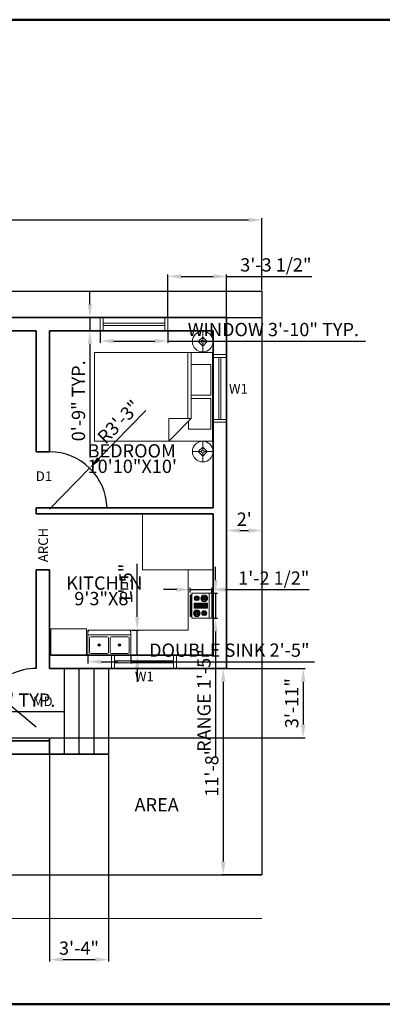
# Model space of a CAD drawing. Units: inches. Extents: x 2113 to 4530, y 1685 to 2353.
# Tile 4 of 6: x 2591 to 2836, y 1685 to 2353. Entities that reach past the tile are written whole.
import ezdxf

# ---------------------------------------------------------------- set-up
doc = ezdxf.new("R2010")
doc.units = ezdxf.units.IN
for name, color, linetype, lineweight in [('A-ANNO-DIMS', 2, 'Continuous', 18), ('A-ANNO-TEXT', 7, 'Continuous', 18), ('A-ANNO-TTLB', 7, 'Continuous', 50), ('A-AREA-IDEN', 7, 'Continuous', 18), ('A-DOOR', 3, 'Continuous', 25), ('A-EQPM', 9, 'Continuous', 18), ('A-FLOR-CASE', 8, 'Continuous', 18), ('A-FLOR-FIXT', 9, 'Continuous', 18), ('A-FLOR-STRS', 7, 'Continuous', 25), ('A-FURN', 8, 'Continuous', 18), ('A-GLAZ', 4, 'Continuous', 18), ('A-WALL', 7, 'Continuous', 35), ('C-PROP', 7, 'Continuous', 25), ('C-ROAD', 8, 'Continuous', 18), ('S-ANNO-DIMS', 2, 'Continuous', 18)]:
    doc.layers.add(name, color=color, linetype=linetype, lineweight=lineweight)
doc.styles.get("Standard").update_dxf_attribs({"font": 'arial.ttf'})
doc.dimstyles.new('ISO-25', dxfattribs={"dimtxt": 9, "dimasz": 9, "dimexe": 1.25, "dimexo": 0.625, "dimgap": 2, "dimtad": 1, "dimdec": 1, "dimlunit": 4, "dimtxsty": 'Standard', "dimcen": 2.5, "dimazin": 0, "dimtfac": 1, "dimtdec": 1, "dimtmove": 0, "dimatfit": 3, "dimfxl": 1, "dimarcsym": 0})

# ---------------------------------------------------------------- blocks, each defined once
blk = doc.blocks.new('Bed - Queen')
for p, q in [((0, -80.00003), (0, 0)), ((0, 0), (59.99999, 0)), ((59.99999, 0), (59.99999, -80.00003)), ((7.99999, -1.2), (28.79998, -1.2)), ((7.99999, -14.4), (7.99999, -1.2)), ((28.79998, -1.2), (28.79998, -14.4)), ((31.19999, -1.2), (51.99999, -1.2)), ((31.19999, -14.4), (31.19999, -1.2)), ((51.99999, -1.2), (51.99999, -16.4)), ((0, -14.4), (44.8, -14.4)), ((44.8, -16.8), (0, -16.8)), ((59.99999, -29.6), (44.8, -14.4)), ((44.8, -14.4), (44.8, -29.6)), ((51.99999, -16.4), (46.79936, -16.4)), ((44.8, -29.6), (59.99999, -29.6)), ((59.99999, -80.00003), (0, -80.00003))]:
    blk.add_line(p, q)
blk = doc.blocks.new('Range-Oven - 30 in top')
for p, q in [((0, -3), (30, -3)), ((12, -6), (18, -6)), ((13, -20), (13, -6)), ((14, -6), (14, -20)), ((15, -20), (15, -6)), ((16, -6), (16, -20)), ((17, -20), (17, -6)), ((18, -20), (12, -20)), ((6, -24), (6, -25)), ((8, -25), (8, -24)), ((22, -25), (22, -24)), ((24, -24), (24, -25))]:
    blk.add_line(p, q)
for points in [[(0, -24), (0, 0), (30, 0), (30, -24)], [(12, -21), (12, -5), (18, -5), (18, -21)], [(2, -26), (2, -25), (28, -25), (28, -26)]]:
    blk.add_lwpolyline(points, close=True)
for centre, radius in [((6, -9), 4), ((6, -9), 3), ((6, -9), 2), ((6, -9), 1), ((24, -9), 3), ((24, -9), 2), ((24, -9), 1), ((6, -18), 3), ((6, -18), 2), ((6, -18), 1), ((24, -18), 4), ((24, -18), 3), ((24, -18), 2), ((24, -18), 1)]:
    blk.add_circle(centre, radius)
blk = doc.blocks.new('Sink-double - 36 in top')
for p, q in [((-18, -4), (18, -4)), ((-0.75, -18.5), (-0.75, -6.5)), ((0.75, -6.5), (0.75, -18.5))]:
    blk.add_line(p, q)
for points in [[(-16.5, 0), (16.5, 0)], [(-18, -19.5), (-18, -1.5)], [(-16.5, -18.5), (-16.5, -6.5)], [(-15.5, -5.5), (-1.75, -5.5)], [(1.75, -5.5), (15.5, -5.5)], [(16.5, -6.5), (16.5, -18.5)], [(18, -1.5), (18, -19.5)], [(16.5, -21), (-16.5, -21)], [(-1.75, -19.5), (-15.5, -19.5)], [(15.5, -19.5), (1.75, -19.5)]]:
    blk.add_lwpolyline(points)
for centre, radius in [((-8.5, -12.5), 1), ((-8.5, -12.5), 0.5), ((8.5, -12.5), 1), ((8.5, -12.5), 0.5)]:
    blk.add_circle(centre, radius)
for centre, radius, start, end in [((-16.5, -1.5), 1.5, 90, 180), ((16.5, -1.5), 1.5, 0, 90), ((-15.5, -6.5), 1, 90, 180), ((-1.75, -6.5), 1, 0, 90), ((1.75, -6.5), 1, 90, 180), ((15.5, -6.5), 1, 0, 90), ((-16.5, -19.5), 1.5, 180, 270), ((-15.5, -18.5), 1, 180, 270), ((-1.75, -18.5), 1, 270, 0), ((1.75, -18.5), 1, 180, 270), ((15.5, -18.5), 1, 270, 0), ((16.5, -19.5), 1.5, 270, 0)]:
    blk.add_arc(centre, radius, start, end)
blk = doc.blocks.new('Lamp - Table')
for p, q in [((0, 7), (0, 1)), ((-1, 0), (-7, 0)), ((0, 3), (-3, 0)), ((-3, 0), (0, -3)), ((3, 0), (0, 3)), ((0, -3), (3, 0)), ((1, 0), (7, 0)), ((0, -1), (0, -7))]:
    blk.add_line(p, q)
for radius in [7, 1]:
    blk.add_circle((0, 0), radius)
blk = doc.blocks.new('*D7')
at = {"layer": 'A-ANNO-DIMS', "color": 0, "lineweight": -2, "transparency": 16777216}
for p, q in [((2289.73, 2169.51), (2289.73, 2218.38)), ((2754.73, 2169.51), (2754.73, 2218.38)), ((2298.73, 2217.13), (2745.73, 2217.13))]:
    blk.add_line(p, q, dxfattribs=at)
at = {"layer": 'A-ANNO-DIMS', "color": 0, "transparency": 16777216}
for points in [[(2298.73, 2218.63), (2298.73, 2215.63), (2289.73, 2217.13)], [(2745.73, 2218.63), (2745.73, 2215.63), (2754.73, 2217.13)]]:
    blk.add_solid(points, dxfattribs=at)
at = {"layer": 'Defpoints', "color": 0, "transparency": 16777216}
for p in [(2754.73, 2217.13), (2289.73, 2168.89), (2754.73, 2168.89)]:
    blk.add_point(p, dxfattribs=at)
at = {"layer": 'A-ANNO-DIMS', "color": 0, "transparency": 16777216, "insert": (2522.23, 2223.73), "char_height": 9, "attachment_point": 5}
blk.add_mtext('38\'-9"', dxfattribs=at)
blk = doc.blocks.new('*D25')
at = {"layer": 'A-ANNO-DIMS', "color": 0, "lineweight": -2, "transparency": 16777216}
for p, q in [((2730.73, 2150.26), (2730.73, 2005.22)), ((2754.73, 2150.26), (2754.73, 2005.22)), ((2739.73, 2006.47), (2745.73, 2006.47))]:
    blk.add_line(p, q, dxfattribs=at)
at = {"layer": 'A-ANNO-DIMS', "color": 0, "transparency": 16777216}
for points in [[(2739.73, 2007.97), (2739.73, 2004.97), (2730.73, 2006.47)], [(2745.73, 2007.97), (2745.73, 2004.97), (2754.73, 2006.47)]]:
    blk.add_solid(points, dxfattribs=at)
at = {"layer": 'Defpoints', "color": 0, "transparency": 16777216}
for p in [(2730.73, 2150.89), (2754.73, 2150.89), (2754.73, 2006.47)]:
    blk.add_point(p, dxfattribs=at)
at = {"layer": 'A-ANNO-DIMS', "color": 0, "transparency": 16777216, "insert": (2742.73, 2012.99), "char_height": 9, "attachment_point": 5}
blk.add_mtext("2'", dxfattribs=at)
blk = doc.blocks.new('*D27')
at = {"layer": 'A-ANNO-DIMS', "color": 0, "lineweight": -2, "transparency": 16777216}
for p, q in [((2730.11, 1912.89), (2727.25, 1912.89)), ((2728.5, 1903.89), (2728.5, 1781.89)), ((2754.11, 1772.89), (2727.25, 1772.89))]:
    blk.add_line(p, q, dxfattribs=at)
at = {"layer": 'A-ANNO-DIMS', "color": 0, "transparency": 16777216}
for points in [[(2727, 1903.89), (2730, 1903.89), (2728.5, 1912.89)], [(2727, 1781.89), (2730, 1781.89), (2728.5, 1772.89)]]:
    blk.add_solid(points, dxfattribs=at)
at = {"layer": 'Defpoints', "color": 0, "transparency": 16777216}
for p in [(2730.73, 1912.89), (2728.5, 1772.89), (2754.73, 1772.89)]:
    blk.add_point(p, dxfattribs=at)
at = {"layer": 'A-ANNO-DIMS', "color": 0, "transparency": 16777216, "insert": (2721.91, 1842.89), "char_height": 9, "attachment_point": 5, "rotation": 90}
blk.add_mtext('11\'-8"', dxfattribs=at)
blk = doc.blocks.new('WINDOW-46')
for p, q in [((0, 46), (9, 46)), ((0, 44), (9, 44)), ((3.75, 44), (3.75, 2)), ((5.25, 44), (5.25, 2)), ((0, 2), (9, 2)), ((0, 0), (9, 0))]:
    blk.add_line(p, q)
blk = doc.blocks.new('LOT-465X396')
for p, q in [((0, 396), (465, 396)), ((0, 396), (0, 0)), ((465, 396), (465, 0)), ((0, 0), (465, 0))]:
    blk.add_line(p, q)
blk = doc.blocks.new('*D50')
at = {"layer": 'Defpoints', "color": 0, "transparency": 16777216}
for p in [(2462.73, 1885.89), (2477.73, 1885.89), (2477.73, 1883.64)]:
    blk.add_point(p, dxfattribs=at)
at = {"layer": 'S-ANNO-DIMS', "color": 0, "lineweight": -2, "transparency": 16777216}
for p, q in [((2453.73, 1883.64), (2444.73, 1883.64)), ((2462.73, 1885.26), (2462.73, 1882.39)), ((2462.73, 1883.64), (2477.73, 1883.64)), ((2477.73, 1885.26), (2477.73, 1882.39)), ((2486.73, 1883.64), (2620.23, 1883.64))]:
    blk.add_line(p, q, dxfattribs=at)
at = {"layer": 'S-ANNO-DIMS', "color": 0, "transparency": 16777216}
for points in [[(2453.73, 1885.14), (2453.73, 1882.14), (2462.73, 1883.64)], [(2486.73, 1885.14), (2486.73, 1882.14), (2477.73, 1883.64)]]:
    blk.add_solid(points, dxfattribs=at)
at = {"layer": 'S-ANNO-DIMS', "color": 0, "transparency": 16777216, "insert": (2557.98, 1890.29), "char_height": 9, "attachment_point": 5}
blk.add_mtext('SEAT PAD 1\'-3" TYP.', dxfattribs=at)
blk = doc.blocks.new('*D56')
at = {"layer": 'Defpoints', "color": 0, "transparency": 16777216}
for p in [(2645.03, 2141.89), (2691.03, 2141.89), (2691.03, 2134.99)]:
    blk.add_point(p, dxfattribs=at)
at = {"layer": 'S-ANNO-DIMS', "color": 0, "lineweight": -2, "transparency": 16777216}
for p, q in [((2645.03, 2141.26), (2645.03, 2133.74)), ((2691.03, 2141.26), (2691.03, 2133.74)), ((2654.03, 2134.99), (2682.03, 2134.99)), ((2691.03, 2134.99), (2824.91, 2134.99))]:
    blk.add_line(p, q, dxfattribs=at)
at = {"layer": 'S-ANNO-DIMS', "color": 0, "transparency": 16777216}
for points in [[(2654.03, 2136.49), (2654.03, 2133.49), (2645.03, 2134.99)], [(2682.03, 2136.49), (2682.03, 2133.49), (2691.03, 2134.99)]]:
    blk.add_solid(points, dxfattribs=at)
at = {"layer": 'S-ANNO-DIMS', "color": 0, "transparency": 16777216, "insert": (2762.47, 2141.65), "char_height": 9, "attachment_point": 5}
blk.add_mtext('WINDOW 3\'-10" TYP.', dxfattribs=at)
blk = doc.blocks.new('*D57')
at = {"layer": 'Defpoints', "color": 0, "transparency": 16777216}
for p in [(2645.03, 2150.89), (2638.13, 2141.89), (2645.03, 2141.89)]:
    blk.add_point(p, dxfattribs=at)
at = {"layer": 'S-ANNO-DIMS', "color": 0, "lineweight": -2, "transparency": 16777216}
for p, q in [((2638.13, 2159.89), (2638.13, 2168.89)), ((2644.4, 2150.89), (2636.88, 2150.89)), ((2638.13, 2150.89), (2638.13, 2141.89)), ((2644.4, 2141.89), (2636.88, 2141.89)), ((2638.13, 2132.89), (2638.13, 2065.03))]:
    blk.add_line(p, q, dxfattribs=at)
at = {"layer": 'S-ANNO-DIMS', "color": 0, "transparency": 16777216}
for points in [[(2636.63, 2159.89), (2639.63, 2159.89), (2638.13, 2150.89)], [(2636.63, 2132.89), (2639.63, 2132.89), (2638.13, 2141.89)]]:
    blk.add_solid(points, dxfattribs=at)
at = {"layer": 'S-ANNO-DIMS', "color": 0, "transparency": 16777216, "insert": (2631.53, 2094.46), "char_height": 9, "attachment_point": 5, "rotation": 90}
blk.add_mtext('0\'-9" TYP.', dxfattribs=at)
blk = doc.blocks.new('*D60')
at = {"layer": 'Defpoints', "color": 0, "transparency": 16777216}
for p in [(2720.73, 1963.89), (2720.73, 1946.95), (2723.27, 1946.95)]:
    blk.add_point(p, dxfattribs=at)
at = {"layer": 'S-ANNO-DIMS', "color": 0, "lineweight": -2, "transparency": 16777216}
for p, q in [((2723.27, 1972.89), (2723.27, 1981.89)), ((2721.35, 1963.89), (2724.52, 1963.89)), ((2723.27, 1963.89), (2723.27, 1946.95)), ((2721.35, 1946.95), (2724.52, 1946.95)), ((2723.27, 1937.95), (2723.27, 1853.29))]:
    blk.add_line(p, q, dxfattribs=at)
at = {"layer": 'S-ANNO-DIMS', "color": 0, "transparency": 16777216}
for points in [[(2721.77, 1972.89), (2724.77, 1972.89), (2723.27, 1963.89)], [(2721.77, 1937.95), (2724.77, 1937.95), (2723.27, 1946.95)]]:
    blk.add_solid(points, dxfattribs=at)
at = {"layer": 'S-ANNO-DIMS', "color": 0, "transparency": 16777216, "insert": (2716.62, 1891.12), "char_height": 9, "attachment_point": 5, "rotation": 90}
blk.add_mtext('RANGE 1\'-5"', dxfattribs=at)
blk = doc.blocks.new('*D61')
at = {"layer": 'Defpoints', "color": 0, "transparency": 16777216}
for p in [(2706.05, 1963.89), (2720.73, 1966.43), (2720.73, 1963.89)]:
    blk.add_point(p, dxfattribs=at)
at = {"layer": 'S-ANNO-DIMS', "color": 0, "lineweight": -2, "transparency": 16777216}
for p, q in [((2697.05, 1966.43), (2688.05, 1966.43)), ((2706.05, 1964.51), (2706.05, 1967.68)), ((2706.05, 1966.43), (2720.73, 1966.43)), ((2720.73, 1964.51), (2720.73, 1967.68)), ((2729.73, 1966.43), (2786.78, 1966.43))]:
    blk.add_line(p, q, dxfattribs=at)
at = {"layer": 'S-ANNO-DIMS', "color": 0, "transparency": 16777216}
for points in [[(2697.05, 1967.93), (2697.05, 1964.93), (2706.05, 1966.43)], [(2729.73, 1967.93), (2729.73, 1964.93), (2720.73, 1966.43)]]:
    blk.add_solid(points, dxfattribs=at)
at = {"layer": 'S-ANNO-DIMS', "color": 0, "transparency": 16777216, "insert": (2762.75, 1973.08), "char_height": 9, "attachment_point": 5}
blk.add_mtext('1\'-2 1/2"', dxfattribs=at)
blk = doc.blocks.new('*D62')
at = {"layer": 'Defpoints', "color": 0, "transparency": 16777216}
for p in [(2636.73, 1921.89), (2665.87, 1921.89), (2665.87, 1917.52)]:
    blk.add_point(p, dxfattribs=at)
at = {"layer": 'S-ANNO-DIMS', "color": 0, "lineweight": -2, "transparency": 16777216}
for p, q in [((2636.73, 1921.26), (2636.73, 1916.27)), ((2645.73, 1917.52), (2656.87, 1917.52)), ((2665.87, 1921.26), (2665.87, 1916.27)), ((2665.87, 1917.52), (2790.38, 1917.52))]:
    blk.add_line(p, q, dxfattribs=at)
at = {"layer": 'S-ANNO-DIMS', "color": 0, "transparency": 16777216}
for points in [[(2645.73, 1919.02), (2645.73, 1916.02), (2636.73, 1917.52)], [(2656.87, 1919.02), (2656.87, 1916.02), (2665.87, 1917.52)]]:
    blk.add_solid(points, dxfattribs=at)
at = {"layer": 'S-ANNO-DIMS', "color": 0, "transparency": 16777216, "insert": (2732.63, 1924.17), "char_height": 9, "attachment_point": 5}
blk.add_mtext('DOUBLE SINK 2\'-5"', dxfattribs=at)
blk = doc.blocks.new('*D63')
at = {"layer": 'Defpoints', "color": 0, "transparency": 16777216}
for p in [(2665.87, 1938.89), (2670.24, 1938.89), (2665.87, 1921.89)]:
    blk.add_point(p, dxfattribs=at)
at = {"layer": 'S-ANNO-DIMS', "color": 0, "lineweight": -2, "transparency": 16777216}
for p, q in [((2670.24, 1947.89), (2670.24, 1983.96)), ((2666.5, 1938.89), (2671.49, 1938.89)), ((2670.24, 1921.89), (2670.24, 1938.89)), ((2666.5, 1921.89), (2671.49, 1921.89)), ((2670.24, 1912.89), (2670.24, 1903.89))]:
    blk.add_line(p, q, dxfattribs=at)
at = {"layer": 'S-ANNO-DIMS', "color": 0, "transparency": 16777216}
for points in [[(2668.74, 1947.89), (2671.74, 1947.89), (2670.24, 1938.89)], [(2668.74, 1912.89), (2671.74, 1912.89), (2670.24, 1921.89)]]:
    blk.add_solid(points, dxfattribs=at)
at = {"layer": 'S-ANNO-DIMS', "color": 0, "transparency": 16777216, "insert": (2663.65, 1970.42), "char_height": 9, "attachment_point": 5, "rotation": 90}
blk.add_mtext('1\'-5"', dxfattribs=at)
blk = doc.blocks.new('*D91')
at = {"layer": 'Defpoints', "color": 0, "transparency": 16777216}
for p in [(2610.73, 1854.89), (2650.73, 1854.89), (2650.73, 1715.45)]:
    blk.add_point(p, dxfattribs=at)
at = {"layer": 'S-ANNO-DIMS', "color": 0, "lineweight": -2, "transparency": 16777216}
for p, q in [((2610.73, 1854.26), (2610.73, 1714.2)), ((2650.73, 1854.26), (2650.73, 1714.2)), ((2619.73, 1715.45), (2641.73, 1715.45))]:
    blk.add_line(p, q, dxfattribs=at)
at = {"layer": 'S-ANNO-DIMS', "color": 0, "transparency": 16777216}
for points in [[(2619.73, 1716.95), (2619.73, 1713.95), (2610.73, 1715.45)], [(2641.73, 1716.95), (2641.73, 1713.95), (2650.73, 1715.45)]]:
    blk.add_solid(points, dxfattribs=at)
at = {"layer": 'S-ANNO-DIMS', "color": 0, "transparency": 16777216, "insert": (2630.73, 1722.05), "char_height": 9, "attachment_point": 5}
blk.add_mtext('3\'-4"', dxfattribs=at)
blk = doc.blocks.new('*D92')
at = {"layer": 'Defpoints', "color": 0, "transparency": 16777216}
for p in [(2610.73, 1912.89), (2610.73, 1865.89), (2782.68, 1865.89)]:
    blk.add_point(p, dxfattribs=at)
at = {"layer": 'S-ANNO-DIMS', "color": 0, "lineweight": -2, "transparency": 16777216}
for p, q in [((2611.36, 1912.89), (2783.93, 1912.89)), ((2782.68, 1903.89), (2782.68, 1874.89)), ((2611.36, 1865.89), (2783.93, 1865.89))]:
    blk.add_line(p, q, dxfattribs=at)
at = {"layer": 'S-ANNO-DIMS', "color": 0, "transparency": 16777216}
for points in [[(2781.18, 1903.89), (2784.18, 1903.89), (2782.68, 1912.89)], [(2781.18, 1874.89), (2784.18, 1874.89), (2782.68, 1865.89)]]:
    blk.add_solid(points, dxfattribs=at)
at = {"layer": 'S-ANNO-DIMS', "color": 0, "transparency": 16777216, "insert": (2776.08, 1889.39), "char_height": 9, "attachment_point": 5, "rotation": 90}
blk.add_mtext('3\'-11"', dxfattribs=at)
blk = doc.blocks.new('*D101')
at = {"layer": 'Defpoints', "color": 0, "transparency": 16777216}
for p in [(2730.73, 2178.84), (2691.03, 2150.89), (2730.73, 2150.89)]:
    blk.add_point(p, dxfattribs=at)
at = {"layer": 'S-ANNO-DIMS', "color": 0, "lineweight": -2, "transparency": 16777216}
for p, q in [((2691.03, 2151.51), (2691.03, 2180.09)), ((2700.03, 2178.84), (2721.73, 2178.84)), ((2730.73, 2151.51), (2730.73, 2180.09)), ((2730.73, 2178.84), (2788.62, 2178.84))]:
    blk.add_line(p, q, dxfattribs=at)
at = {"layer": 'S-ANNO-DIMS', "color": 0, "transparency": 16777216}
for points in [[(2700.03, 2180.34), (2700.03, 2177.34), (2691.03, 2178.84)], [(2721.73, 2180.34), (2721.73, 2177.34), (2730.73, 2178.84)]]:
    blk.add_solid(points, dxfattribs=at)
at = {"layer": 'S-ANNO-DIMS', "color": 0, "transparency": 16777216, "insert": (2764.18, 2185.49), "char_height": 9, "attachment_point": 5}
blk.add_mtext('3\'-3 1/2"', dxfattribs=at)
blk = doc.blocks.new('*D102')
at = {"layer": 'Defpoints', "color": 0, "transparency": 16777216}
for p in [(2571.2, 1898.54), (2601.73, 1873.2)]:
    blk.add_point(p, dxfattribs=at)
at = {"layer": 'S-ANNO-DIMS', "color": 0, "lineweight": -2, "transparency": 16777216}
for p, q in [((2513.09, 1946.76), (2564.27, 1904.29)), ((2601.73, 1873.2), (2571.2, 1898.54))]:
    blk.add_line(p, q, dxfattribs=at)
at = {"layer": 'S-ANNO-DIMS', "color": 0, "transparency": 16777216}
blk.add_solid([(2565.23, 1905.45), (2563.31, 1903.14), (2571.2, 1898.54)], dxfattribs=at)
at = {"layer": 'S-ANNO-DIMS', "color": 0, "transparency": 16777216, "insert": (2539.47, 1933.52), "char_height": 9, "attachment_point": 5, "rotation": 320.31503}
blk.add_mtext('R3\'-3 1/2"', dxfattribs=at)
blk = doc.blocks.new('*D103')
at = {"layer": 'Defpoints', "color": 0, "transparency": 16777216}
for p in [(2637.96, 2048.82), (2610.73, 2020.87)]:
    blk.add_point(p, dxfattribs=at)
at = {"layer": 'S-ANNO-DIMS', "color": 0, "lineweight": -2, "transparency": 16777216}
for p, q in [((2676.02, 2087.88), (2644.24, 2055.26)), ((2610.73, 2020.87), (2637.96, 2048.82))]:
    blk.add_line(p, q, dxfattribs=at)
at = {"layer": 'S-ANNO-DIMS', "color": 0, "transparency": 16777216}
blk.add_solid([(2643.16, 2056.31), (2645.31, 2054.21), (2637.96, 2048.82)], dxfattribs=at)
at = {"layer": 'S-ANNO-DIMS', "color": 0, "transparency": 16777216, "insert": (2658.54, 2079.4), "char_height": 9, "attachment_point": 5, "rotation": 45.7443}
blk.add_mtext('R3\'-3"', dxfattribs=at)

msp = doc.modelspace()

# ---------------------------------------------------------------- linework, layer by layer
at = {"layer": 'A-ANNO-TTLB'}
msp.add_lwpolyline([(2112.77, 2352.97), (4498.42, 2352.97), (4498.42, 1685.12), (2112.77, 1685.12)], close=True, dxfattribs=at)
at = {"layer": 'A-DOOR'}
msp.add_line((2562.73, 1865.89), (2610.73, 1865.89), dxfattribs=at)
for centre, radius, start, end in [((2610.73, 2020.87), 39.01, 1.48812, 90), ((2601.73, 1873.2), 39.68, 90, 190.62909)]:
    msp.add_arc(centre, radius, start, end, dxfattribs=at)
at = {"layer": 'A-FLOR-CASE'}
for p, q in [((2673.73, 2017.89), (2673.73, 1979.89)), ((2673.73, 1979.89), (2721.73, 1979.89)), ((2704.73, 1979.89), (2704.73, 1938.89)), ((2611.73, 1939.89), (2635.73, 1939.89)), ((2611.73, 1939.89), (2611.73, 1921.89)), ((2635.73, 1939.89), (2635.73, 1921.89)), ((2636.73, 1938.89), (2704.73, 1938.89)), ((2636.73, 1938.89), (2636.73, 1921.89)), ((2611.73, 1921.89), (2635.73, 1921.89))]:
    msp.add_line(p, q, dxfattribs=at)
at = {"layer": 'A-FLOR-STRS'}
for p, q in [((2620.73, 1912.89), (2620.73, 1854.89)), ((2630.73, 1912.89), (2630.73, 1854.89)), ((2640.73, 1912.89), (2640.73, 1854.89)), ((2650.73, 1912.89), (2650.73, 1854.89))]:
    msp.add_line(p, q, dxfattribs=at)
at = {"layer": 'A-GLAZ'}
for p, q in [((2652.73, 1921.89), (2652.73, 1912.89)), ((2654.73, 1921.89), (2654.73, 1912.89)), ((2654.73, 1918.14), (2694.73, 1918.14)), ((2694.73, 1921.89), (2694.73, 1912.89)), ((2696.73, 1921.89), (2696.73, 1912.89)), ((2654.73, 1916.64), (2694.73, 1916.64))]:
    msp.add_line(p, q, dxfattribs=at)
at = {"layer": 'A-WALL'}
for p, q in [((2313.73, 2150.89), (2730.73, 2150.89)), ((2730.73, 2150.89), (2730.73, 1912.89)), ((2563.73, 2141.89), (2601.73, 2141.89)), ((2601.73, 2141.89), (2601.73, 2059.89)), ((2610.73, 2141.89), (2610.73, 2059.89)), ((2610.73, 2141.89), (2721.73, 2141.89)), ((2721.73, 2141.89), (2721.73, 2021.89)), ((2601.73, 2059.89), (2610.73, 2059.89)), ((2601.73, 2021.89), (2721.73, 2021.89)), ((2601.73, 2021.89), (2601.73, 2017.89)), ((2601.73, 2017.89), (2721.73, 2017.89)), ((2721.73, 2017.89), (2721.73, 1921.89)), ((2601.73, 1979.89), (2610.73, 1979.89)), ((2601.73, 1979.89), (2601.73, 1912.89)), ((2610.73, 1979.89), (2610.73, 1912.89)), ((2611.73, 1921.89), (2721.73, 1921.89)), ((2610.73, 1912.89), (2730.73, 1912.89)), ((2456.73, 1863.89), (2610.73, 1863.89)), ((2610.73, 1865.89), (2610.73, 1854.89)), ((2322.73, 1854.89), (2650.73, 1854.89))]:
    msp.add_line(p, q, dxfattribs=at)
at = {"layer": 'C-PROP'}
msp.add_line((2730.73, 2150.89), (2754.73, 2150.89), dxfattribs=at)
at = {"layer": 'C-ROAD'}
msp.add_line((2314.56, 1743.4), (2754.73, 1743.4), dxfattribs=at)

# ---------------------------------------------------------------- block references
at = {"layer": 'A-EQPM', "xscale": 0.5645220266747233, "yscale": 0.5645220266747233, "zscale": 0.5645220266747233, "rotation": 269.9999999999999}
msp.add_blockref('Range-Oven - 30 in top', (2720.73, 1963.89), dxfattribs=at)
at = {"layer": 'A-FLOR-FIXT', "xscale": 0.8093854898181806, "yscale": 0.8093854898181806, "zscale": 0.8093854898181806}
msp.add_blockref('Sink-double - 36 in top', (2651.3, 1938.89), dxfattribs=at)
at = {"layer": 'A-FURN'}
for p in [(2714.6, 2134.61), (2714.6, 2060.01)]:
    msp.add_blockref('Lamp - Table', p, dxfattribs=at)
at = {"layer": 'A-FURN', "rotation": 269.9999999999999}
msp.add_blockref('Bed - Queen', (2721.26, 2127.19), dxfattribs=at)
at = {"layer": 'A-GLAZ', "rotation": 270}
msp.add_blockref('WINDOW-46', (2645.03, 2150.89), dxfattribs=at)
at = {"layer": 'A-GLAZ'}
msp.add_blockref('WINDOW-46', (2721.73, 2079.89), dxfattribs=at)
at = {"layer": 'C-PROP'}
msp.add_blockref('LOT-465X396', (2289.73, 1772.89), dxfattribs=at)

# ---------------------------------------------------------------- texts
at = {"layer": 'A-ANNO-TEXT'}
for s, p in [('W1', (2732.4, 2099.39)), (' D1', (2599.48, 2040.06)), ('W1', (2668.63, 1904.21)), ('MD', (2599.48, 1887.35))]:
    msp.add_text(s, height=6.54, dxfattribs=at).set_placement(p)
msp.add_text(' ARCH', height=6.54, rotation=90, dxfattribs=at).set_placement((2609.72, 1983.01))
at = {"layer": 'A-AREA-IDEN'}
for s, p in [('   BEDROOM', (2628.32, 2056.03)), ('   10\'10"X10\'', (2628.32, 2045.53)), ('    KITCHEN', (2611.05, 1966.34)), ('      9\'3"X8\'', (2611.05, 1955.83)), ('       AREA', (2649.15, 1815.96))]:
    msp.add_text(s, height=9, dxfattribs=at).set_placement(p)

# ---------------------------------------------------------------- dimensions: what is measured, and where the dimension line sits
at = {"layer": 'A-ANNO-DIMS'}
for base, p1, p2, picture, middle in [((2754.73, 2217.13), (2289.73, 2168.89), (2754.73, 2168.89), '*D7', (2522.23, 2223.73)), ((2754.73, 2006.47), (2730.73, 2150.89), (2754.73, 2150.89), '*D25', (2742.73, 2012.99))]:
    dim = msp.add_linear_dim(base=base, p1=p1, p2=p2, dimstyle='ISO-25', override={"dimclrd": 0, "dimclre": 0, "dimclrt": 0}, dxfattribs=at)
    dim.commit()
    dim.dimension.update_dxf_attribs({"geometry": picture, "text_midpoint": middle})
dim = msp.add_linear_dim(base=(2728.5, 1772.89), p1=(2730.73, 1912.89), p2=(2754.73, 1772.89), angle=90, dimstyle='ISO-25', override={"dimclrd": 0, "dimclre": 0, "dimclrt": 0}, dxfattribs=at)
dim.commit()
dim.dimension.update_dxf_attribs({"geometry": '*D27', "text_midpoint": (2721.91, 1842.89)})
at = {"layer": 'S-ANNO-DIMS'}
for base, p1, p2, picture, middle in [((2730.73, 2178.84), (2691.03, 2150.89), (2730.73, 2150.89), '*D101', (2764.18, 2185.49)), ((2720.73, 1966.43), (2706.05, 1963.89), (2720.73, 1963.89), '*D61', (2762.75, 1973.08)), ((2650.73, 1715.45), (2610.73, 1854.89), (2650.73, 1854.89), '*D91', (2630.73, 1722.05))]:
    dim = msp.add_linear_dim(base=base, p1=p1, p2=p2, dimstyle='ISO-25', override={"dimdec": 1, "dimlfac": 1, "dimrnd": 0, "dimzin": 1, "dimdsep": 46, "dimlunit": 4, "dimfrac": 2}, dxfattribs=at)
    dim.commit()
    dim.dimension.update_dxf_attribs({"geometry": picture, "text_midpoint": middle})
for base, p1, p2, text, picture, middle in [((2638.13, 2141.89), (2645.03, 2150.89), (2645.03, 2141.89), '<> TYP.', '*D57', (2631.53, 2094.46)), ((2723.27, 1946.95), (2720.73, 1963.89), (2720.73, 1946.95), 'RANGE <>', '*D60', (2716.62, 1891.12))]:
    dim = msp.add_linear_dim(base=base, p1=p1, p2=p2, angle=270, text=text, dimstyle='ISO-25', override={"dimdec": 1, "dimlfac": 1, "dimrnd": 0, "dimzin": 1, "dimdsep": 46, "dimlunit": 4, "dimfrac": 2}, dxfattribs=at)
    dim.commit()
    dim.dimension.update_dxf_attribs({"geometry": picture, "text_midpoint": middle})
for base, p1, p2, text, picture, middle in [((2691.03, 2134.99), (2645.03, 2141.89), (2691.03, 2141.89), 'WINDOW <> TYP.', '*D56', (2762.47, 2141.65)), ((2665.87, 1917.52), (2636.73, 1921.89), (2665.87, 1921.89), 'DOUBLE SINK <>', '*D62', (2732.63, 1924.17)), ((2477.73, 1883.64), (2462.73, 1885.89), (2477.73, 1885.89), 'SEAT PAD <> TYP.', '*D50', (2557.98, 1890.29))]:
    dim = msp.add_linear_dim(base=base, p1=p1, p2=p2, text=text, dimstyle='ISO-25', override={"dimdec": 1, "dimlfac": 1, "dimrnd": 0, "dimzin": 1, "dimdsep": 46, "dimlunit": 4, "dimfrac": 2}, dxfattribs=at)
    dim.commit()
    dim.dimension.update_dxf_attribs({"geometry": picture, "text_midpoint": middle})
for center, mpoint, picture, middle in [((2610.73, 2020.87), (2637.96, 2048.82), '*D103', (2658.54, 2079.4)), ((2601.73, 1873.2), (2571.2, 1898.54), '*D102', (2539.47, 1933.52))]:
    dim = msp.add_radius_dim(center=center, mpoint=mpoint, dimstyle='ISO-25', override={"dimdec": 1, "dimlfac": 1, "dimrnd": 0, "dimzin": 1, "dimdsep": 46, "dimlunit": 4, "dimfrac": 2}, dxfattribs=at)
    dim.commit()
    dim.dimension.update_dxf_attribs({"geometry": picture, "text_midpoint": middle})
for base, p1, p2, picture, middle in [((2670.24, 1938.89), (2665.87, 1921.89), (2665.87, 1938.89), '*D63', (2663.65, 1970.42)), ((2782.68, 1865.89), (2610.73, 1912.89), (2610.73, 1865.89), '*D92', (2776.08, 1889.39))]:
    dim = msp.add_linear_dim(base=base, p1=p1, p2=p2, angle=90, dimstyle='ISO-25', override={"dimdec": 1, "dimlfac": 1, "dimrnd": 0, "dimzin": 1, "dimdsep": 46, "dimlunit": 4, "dimfrac": 2}, dxfattribs=at)
    dim.commit()
    dim.dimension.update_dxf_attribs({"geometry": picture, "text_midpoint": middle})

doc.saveas('drawing.dxf')
